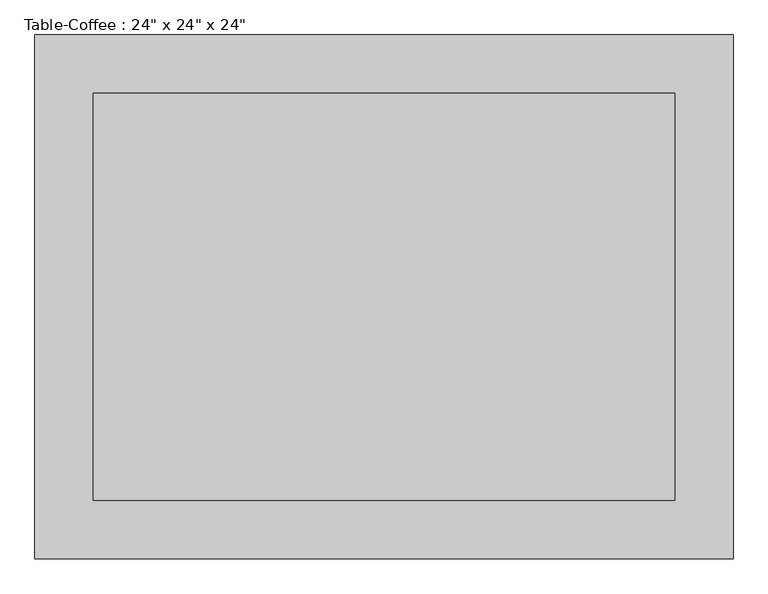
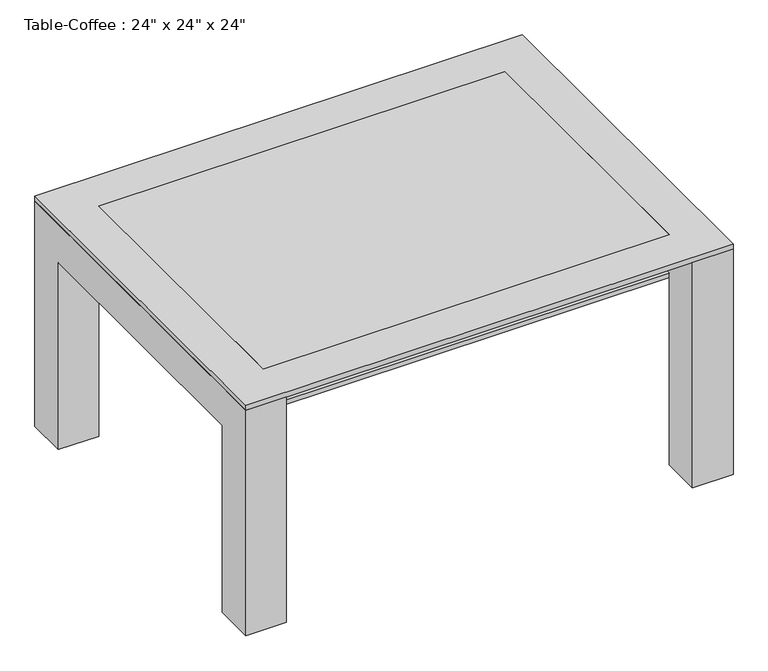
"""IFC4 building model written with IfcOpenShell, lengths in millimetres: furniture geometry."""

from ifc_helpers import new_model, si_unit, frame, origin, place, context, project, spatial, polyline, outline, extrude, source, transform, mapped, element, save


def furniture_4da399da(model_context):
    return source(origin(), model_context, "Body", "SweptSolid", [
        extrude(outline(polyline([(526.2657667, 450.8110778), (526.2657667, -260.3889222), (-489.7342333, -260.3889222), (-489.7342333, 450.8110778), (526.2657667, 450.8110778)])), frame((0.0, 0.0, 495.3), z_axis=(0.0, 0.0, 1.0), x_axis=(1.0, 0.0, 0.0)), (0.0, 0.0, 1.0), 12.7),
        extrude(outline(polyline([(552.4110778, 0.0), (450.8110778, 0.0), (450.8110778, 495.3), (-260.3889222, 495.3), (-260.3889222, 0.0), (-361.9889222, 0.0), (-361.9889222, 596.9), (552.4110778, 596.9), (552.4110778, 0.0)])), frame((526.2657667, 0.0, 0.0), z_axis=(1.0, 0.0, 0.0), x_axis=(0.0, 1.0, 0.0)), (0.0, 0.0, 1.0), 101.6),
        extrude(outline(polyline([(552.4110778, 596.9), (552.4110778, 0.0), (450.8110778, 0.0), (450.8110778, 495.3), (-260.3889222, 495.3), (-260.3889222, 0.0), (-361.9889222, 0.0), (-361.9889222, 596.9), (552.4110778, 596.9)])), frame((-591.3342333, 0.0, 0.0), z_axis=(1.0, 0.0, 0.0), x_axis=(0.0, 1.0, 0.0)), (0.0, 0.0, 1.0), 101.6),
        extrude(outline(polyline([(526.2657667, 450.8110778), (526.2657667, -260.3889222), (-489.7342333, -260.3889222), (-489.7342333, 450.8110778), (526.2657667, 450.8110778)])), frame((0.0, 0.0, 596.9), z_axis=(0.0, 0.0, 1.0), x_axis=(1.0, 0.0, 0.0)), (0.0, 0.0, 1.0), 12.7),
        extrude(outline(polyline([(627.8657667, 552.4110778), (627.8657667, -361.9889222), (-591.3342333, -361.9889222), (-591.3342333, 552.4110778), (627.8657667, 552.4110778)]), holes=[polyline([(526.2657667, 450.8110778), (-489.7342333, 450.8110778), (-489.7342333, -260.3889222), (526.2657667, -260.3889222), (526.2657667, 450.8110778)])]), frame((0.0, 0.0, 596.9), z_axis=(0.0, 0.0, 1.0), x_axis=(1.0, 0.0, 0.0)), (0.0, 0.0, 1.0), 12.7),
    ])


if __name__ == "__main__":
    model = new_model("IFC4")
    model_context = context("Model", 3, world=origin())
    ifc_project = project(units=[si_unit("LENGTHUNIT", "METRE", prefix="MILLI")], contexts=[model_context])
    site = spatial("IfcSite", under=ifc_project)
    building = spatial("IfcBuilding", under=site)
    placement = place(None, origin())
    furniture_shape = furniture_4da399da(model_context)
    element("IfcFurniture", 1, ObjectType="Table-Coffee : 24\" x 24\" x 24\"", at=placement, inside=building, context=model_context, shape_type="MappedRepresentation", body=[
        mapped(furniture_shape, transform((0.0, 0.0, 0.0), x_axis=(1.0, 0.0, 0.0), y_axis=(0.0, 1.0, 0.0), z_axis=(0.0, 0.0, 1.0))),
    ])
    save(model, "model.ifc")

# Revit data of these elements
# Type "Table-Coffee : 24\" x 24\" x 24\""
#   Assembly Code = "E2020200"
#   Height = 2' - 0"
#   Length = 4' - 0"
#   Width = 3' - 0"
#   Top Material = none
#   Frame Material = none
#   Default Elevation = 0
# Element 1 (IfcFurniture, "Table-Coffee : 24\" x 24\" x 24\"")
#   Materials on its faces: "Glass - Clear, Grey"
# Materials
#   "Glass - Clear, Grey": class "Glass", colour RGB 252 255 255, transparency 0.64
